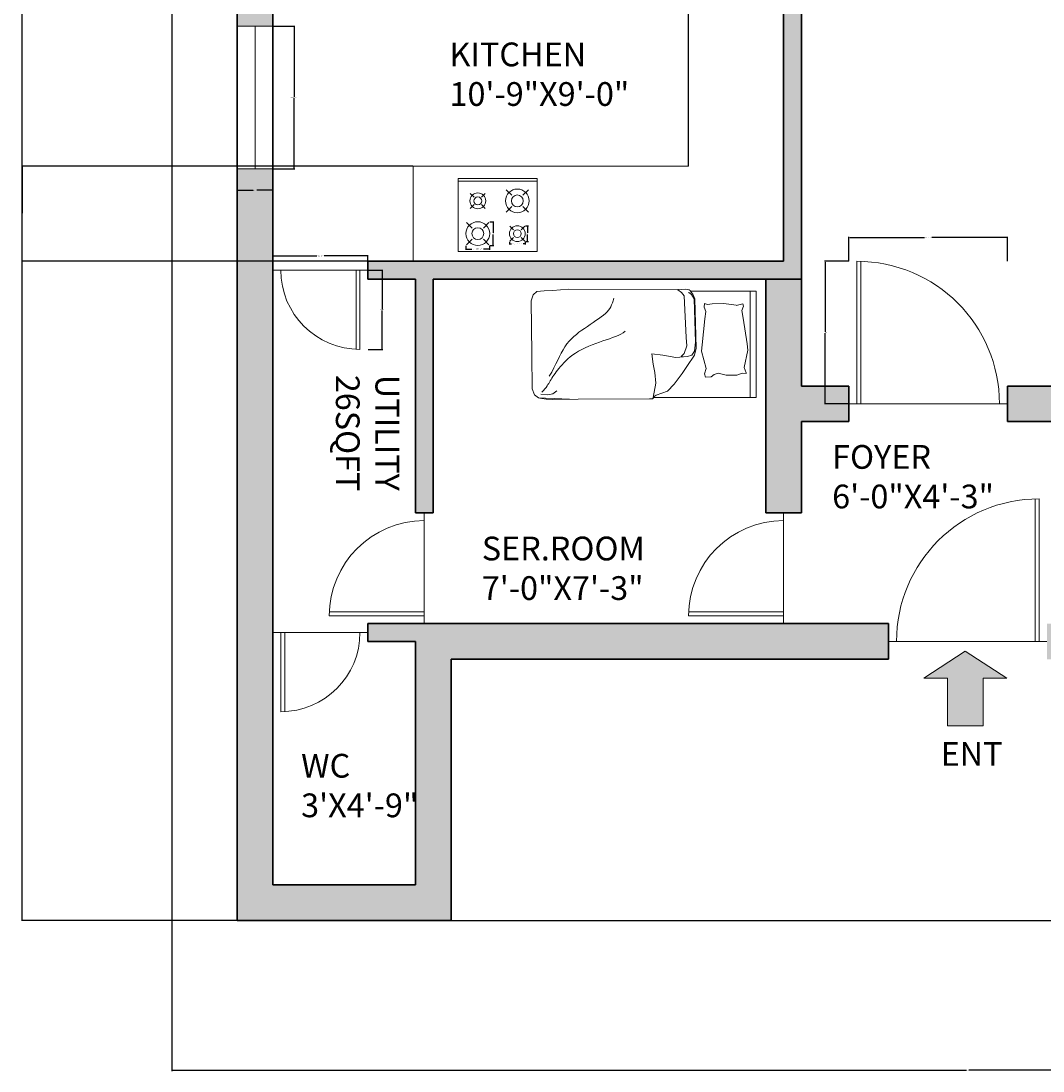
# Model space of a CAD drawing. Units: inches. Extents: x -36 to 442, y -676 to 151.
# Tile 1 of 8: x -36 to 222, y -676 to -411. Entities that reach past the tile are written whole.
import ezdxf

# ---------------------------------------------------------------- set-up
doc = ezdxf.new("R2010")
doc.units = ezdxf.units.IN
doc.header["$MEASUREMENT"] = 0
for name, color, linetype, lineweight in [('A-ANNO-DIMS', 2, 'Continuous', 18), ('A-ANNO-SYMB', 7, 'Continuous', 18), ('A-ANNO-TEXT', 7, 'Continuous', 18), ('A-AREA-IDEN', 7, 'Continuous', 18), ('A-DOOR', 4, 'Continuous', 18), ('A-EQPM', 8, 'Continuous', 18), ('A-FLOR-CASE', 32, 'Continuous', 18), ('A-FURN', 9, 'Continuous', 13), ('A-GLAZ', 4, 'Continuous', 13), ('A-WALL', 7, 'Continuous', 35), ('A-WALL-PATT', 8, 'Continuous', 13)]:
    doc.layers.add(name, color=color, linetype=linetype, lineweight=lineweight)
doc.styles.get("Standard").update_dxf_attribs({"font": 'arial.ttf'})
doc.dimstyles.get("Standard").update_dxf_attribs({"dimtxt": 0.18, "dimasz": 0.18, "dimexe": 0.18, "dimexo": 0.0625, "dimgap": 0.09, "dimtad": 0, "dimtih": 1, "dimtoh": 1, "dimdec": 0, "dimzin": 0, "dimdsep": 46, "dimlunit": 3, "dimtxsty": 'Standard', "dimcen": 0.09, "dimadec": 0, "dimazin": 0, "dimtfac": 1, "dimtdec": 0, "dimtofl": 0, "dimtmove": 0, "dimatfit": 3, "dimfxl": 1, "dimtolj": 1, "dimtzin": 0, "dimarcsym": 0})

# ---------------------------------------------------------------- blocks, each defined once
blk = doc.blocks.new('DOOR-SWING-24IN')
for p, q in [((24, 26), (24, 28)), ((24, 26), (24, 2)), ((24, 3), (0, 3)), ((24, 2), (0, 2)), ((24, 0), (24, 2))]:
    blk.add_line(p, q)
blk.add_arc((24, 2), 24, 90, 180)
blk = doc.blocks.new('DOOR-SWING-36IN')
for p, q in [((2, 0), (2, 36)), ((3, 0), (3, 36)), ((0, 0), (2, 0)), ((2, 0), (3, 0)), ((3, 0), (38, 0)), ((38, 0), (40, 0))]:
    blk.add_line(p, q)
blk.add_arc((2, 0), 36, 0, 90)
blk = doc.blocks.new('DOOR-SWING-20IN')
for p, q in [((0, 20), (2, 20)), ((2, 20), (2, 0)), ((2, 20), (22, 20)), ((3, 20), (3, 0)), ((24, 20), (22, 20))]:
    blk.add_line(p, q)
blk.add_arc((2, 20), 20, 270, 0)
blk = doc.blocks.new('GLAZING-UNIT-36IN')
for p, q in [((0, 36), (0, 0)), ((4.5, 36), (4.5, 0)), ((9, 0), (9, 36))]:
    blk.add_line(p, q)
blk = doc.blocks.new('COOKTOP-BURNER-LARGE')
for p, q in [((1.58, 4.41), (0.17, 5.82)), ((4.41, 4.41), (5.82, 5.82)), ((1.58, 1.58), (0.17, 0.17)), ((4.41, 1.58), (5.82, 0.17))]:
    blk.add_line(p, q)
blk.add_circle((3, 3), 3)
for start, end in [(0, 180), (180, 0)]:
    blk.add_arc((3, 3), 1.5, start, end)
blk = doc.blocks.new('COOKTOP-BURNER-SMALL')
for p, q in [((1.06, 2.94), (0.11, 3.88)), ((2.94, 2.94), (3.88, 3.88)), ((1.06, 1.06), (0.11, 0.11)), ((2.94, 1.06), (3.88, 0.11))]:
    blk.add_line(p, q)
blk.add_circle((2, 2), 2)
for start, end in [(0, 180), (180, 0)]:
    blk.add_arc((2, 2), 0.999, start, end)
blk = doc.blocks.new('*D19')
at = {"layer": 'A-ANNO-DIMS', "color": 0, "lineweight": -2, "transparency": 16777216}
for p, q in [((173.24, -471.43), (173.24, -465.32)), ((173.42, -465.5), (192.3, -465.5)), ((213.06, -465.5), (194.17, -465.5)), ((213.24, -471.43), (213.24, -465.32))]:
    blk.add_line(p, q, dxfattribs=at)
at = {"layer": 'A-ANNO-DIMS', "color": 0, "transparency": 16777216}
for points in [[(173.42, -465.47), (173.42, -465.53), (173.24, -465.5)], [(213.06, -465.47), (213.06, -465.53), (213.24, -465.5)]]:
    blk.add_solid(points, dxfattribs=at)
at = {"layer": 'Defpoints', "color": 0, "transparency": 16777216}
for p in [(213.24, -465.5), (173.24, -471.5), (213.24, -471.5)]:
    blk.add_point(p, dxfattribs=at)
at = {"layer": 'A-ANNO-DIMS', "color": 0, "transparency": 16777216, "insert": (193.24, -465.5), "char_height": 0.18, "attachment_point": 5}
blk.add_mtext('\\A1;DOOR 40 TYP.', dxfattribs=at)
blk = doc.blocks.new('*D20')
at = {"layer": 'A-ANNO-DIMS', "color": 0, "lineweight": -2, "transparency": 16777216}
for p, q in [((173.17, -471.5), (167.06, -471.5)), ((167.24, -471.68), (167.24, -489.32)), ((167.24, -507.32), (167.24, -489.68)), ((173.17, -507.5), (167.06, -507.5))]:
    blk.add_line(p, q, dxfattribs=at)
at = {"layer": 'A-ANNO-DIMS', "color": 0, "transparency": 16777216}
for points in [[(167.21, -471.68), (167.27, -471.68), (167.24, -471.5)], [(167.21, -507.32), (167.27, -507.32), (167.24, -507.5)]]:
    blk.add_solid(points, dxfattribs=at)
at = {"layer": 'Defpoints', "color": 0, "transparency": 16777216}
for p in [(167.24, -471.5), (173.24, -471.5), (173.24, -507.5)]:
    blk.add_point(p, dxfattribs=at)
at = {"layer": 'A-ANNO-DIMS', "color": 0, "transparency": 16777216, "insert": (167.24, -489.5), "char_height": 0.18, "attachment_point": 5}
blk.add_mtext('\\A1;36 TYP.', dxfattribs=at)
blk = doc.blocks.new('*D21')
at = {"layer": 'A-ANNO-DIMS', "color": 0, "lineweight": -2, "transparency": 16777216}
for p, q in [((27.74, -473.68), (27.74, -469.97)), ((27.92, -470.15), (38.8, -470.15)), ((51.56, -470.15), (40.67, -470.15)), ((51.74, -473.68), (51.74, -469.97))]:
    blk.add_line(p, q, dxfattribs=at)
at = {"layer": 'A-ANNO-DIMS', "color": 0, "transparency": 16777216}
for points in [[(27.92, -470.12), (27.92, -470.18), (27.74, -470.15)], [(51.56, -470.12), (51.56, -470.18), (51.74, -470.15)]]:
    blk.add_solid(points, dxfattribs=at)
at = {"layer": 'Defpoints', "color": 0, "transparency": 16777216}
for p in [(27.74, -470.15), (27.74, -473.75), (51.74, -473.75)]:
    blk.add_point(p, dxfattribs=at)
at = {"layer": 'A-ANNO-DIMS', "color": 0, "transparency": 16777216, "insert": (39.74, -470.15), "char_height": 0.18, "attachment_point": 5}
blk.add_mtext('\\A1;DOOR 24 TYP.', dxfattribs=at)
blk = doc.blocks.new('*D22')
at = {"layer": 'A-ANNO-DIMS', "color": 0, "lineweight": -2, "transparency": 16777216}
for p, q in [((51.8, -473.75), (55.52, -473.75)), ((55.34, -473.93), (55.34, -483.57)), ((55.34, -493.57), (55.34, -483.93)), ((51.8, -493.75), (55.52, -493.75))]:
    blk.add_line(p, q, dxfattribs=at)
at = {"layer": 'A-ANNO-DIMS', "color": 0, "transparency": 16777216}
for points in [[(55.31, -473.93), (55.37, -473.93), (55.34, -473.75)], [(55.31, -493.57), (55.37, -493.57), (55.34, -493.75)]]:
    blk.add_solid(points, dxfattribs=at)
at = {"layer": 'Defpoints', "color": 0, "transparency": 16777216}
for p in [(51.74, -473.75), (55.34, -473.75), (51.74, -493.75)]:
    blk.add_point(p, dxfattribs=at)
at = {"layer": 'A-ANNO-DIMS', "color": 0, "transparency": 16777216, "insert": (55.34, -483.75), "char_height": 0.18, "attachment_point": 5}
blk.add_mtext('\\A1;20 TYP.', dxfattribs=at)
blk = doc.blocks.new('*D23')
at = {"layer": 'A-ANNO-DIMS', "color": 0, "lineweight": -2, "transparency": 16777216}
for p, q in [((27.8, -412.15), (33.32, -412.15)), ((33.14, -412.33), (33.14, -429.97)), ((33.14, -447.97), (33.14, -430.33)), ((27.8, -448.15), (33.32, -448.15))]:
    blk.add_line(p, q, dxfattribs=at)
at = {"layer": 'A-ANNO-DIMS', "color": 0, "transparency": 16777216}
for points in [[(33.11, -412.33), (33.17, -412.33), (33.14, -412.15)], [(33.11, -447.97), (33.17, -447.97), (33.14, -448.15)]]:
    blk.add_solid(points, dxfattribs=at)
at = {"layer": 'Defpoints', "color": 0, "transparency": 16777216}
for p in [(27.74, -412.15), (33.14, -412.15), (27.74, -448.15)]:
    blk.add_point(p, dxfattribs=at)
at = {"layer": 'A-ANNO-DIMS', "color": 0, "transparency": 16777216, "insert": (33.14, -430.15), "char_height": 0.18, "attachment_point": 5}
blk.add_mtext('\\A1;WINDOW 36 TYP.', dxfattribs=at)
blk = doc.blocks.new('*D24')
at = {"layer": 'A-ANNO-DIMS', "color": 0, "lineweight": -2, "transparency": 16777216}
for p, q in [((18.74, -448.21), (18.74, -453.73)), ((27.74, -448.21), (27.74, -453.73)), ((18.92, -453.55), (22.78, -453.55)), ((27.56, -453.55), (23.69, -453.55))]:
    blk.add_line(p, q, dxfattribs=at)
at = {"layer": 'A-ANNO-DIMS', "color": 0, "transparency": 16777216}
for points in [[(18.92, -453.52), (18.92, -453.58), (18.74, -453.55)], [(27.56, -453.52), (27.56, -453.58), (27.74, -453.55)]]:
    blk.add_solid(points, dxfattribs=at)
at = {"layer": 'Defpoints', "color": 0, "transparency": 16777216}
for p in [(18.74, -448.15), (27.74, -448.15), (27.74, -453.55)]:
    blk.add_point(p, dxfattribs=at)
at = {"layer": 'A-ANNO-DIMS', "color": 0, "transparency": 16777216, "insert": (23.24, -453.55), "char_height": 0.18, "attachment_point": 5}
blk.add_mtext('\\A1;9 TYP.', dxfattribs=at)
blk = doc.blocks.new('*D33')
at = {"layer": 'A-ANNO-DIMS', "color": 0, "lineweight": -2, "transparency": 16777216}
for p, q in [((76.5, -467.57), (76.5, -468.59)), ((76.68, -468.41), (78.01, -468.41)), ((82.31, -468.41), (80.97, -468.41)), ((82.49, -467.57), (82.49, -468.59))]:
    blk.add_line(p, q, dxfattribs=at)
at = {"layer": 'A-ANNO-DIMS', "color": 0, "transparency": 16777216}
for points in [[(76.68, -468.38), (76.68, -468.44), (76.5, -468.41)], [(82.31, -468.38), (82.31, -468.44), (82.49, -468.41)]]:
    blk.add_solid(points, dxfattribs=at)
at = {"layer": 'Defpoints', "color": 0, "transparency": 16777216}
for p in [(76.5, -467.51), (82.49, -467.51), (82.49, -468.41)]:
    blk.add_point(p, dxfattribs=at)
at = {"layer": 'A-ANNO-DIMS', "color": 0, "transparency": 16777216, "insert": (79.49, -468.41), "char_height": 0.18, "attachment_point": 5}
blk.add_mtext('\\A1;LARGE BURNER 6 TYP.', dxfattribs=at)
blk = doc.blocks.new('*D34')
at = {"layer": 'A-ANNO-DIMS', "color": 0, "lineweight": -2, "transparency": 16777216}
for p, q in [((82.55, -461.52), (83.57, -461.52)), ((83.39, -461.7), (83.39, -464.33)), ((83.39, -467.33), (83.39, -464.7)), ((82.55, -467.51), (83.57, -467.51))]:
    blk.add_line(p, q, dxfattribs=at)
at = {"layer": 'A-ANNO-DIMS', "color": 0, "transparency": 16777216}
for points in [[(83.36, -461.7), (83.42, -461.7), (83.39, -461.52)], [(83.36, -467.33), (83.42, -467.33), (83.39, -467.51)]]:
    blk.add_solid(points, dxfattribs=at)
at = {"layer": 'Defpoints', "color": 0, "transparency": 16777216}
for p in [(82.49, -461.52), (83.39, -461.52), (82.49, -467.51)]:
    blk.add_point(p, dxfattribs=at)
at = {"layer": 'A-ANNO-DIMS', "color": 0, "transparency": 16777216, "insert": (83.39, -464.52), "char_height": 0.18, "attachment_point": 5}
blk.add_mtext('\\A1;6 TYP.', dxfattribs=at)
blk = doc.blocks.new('*D35')
at = {"layer": 'A-ANNO-DIMS', "color": 0, "lineweight": -2, "transparency": 16777216}
for p, q in [((87.48, -466.58), (87.48, -467.29)), ((91.48, -466.58), (91.48, -467.29)), ((87.66, -467.11), (88.01, -467.11)), ((91.3, -467.11), (90.95, -467.11))]:
    blk.add_line(p, q, dxfattribs=at)
at = {"layer": 'A-ANNO-DIMS', "color": 0, "transparency": 16777216}
for points in [[(87.66, -467.08), (87.66, -467.14), (87.48, -467.11)], [(91.3, -467.08), (91.3, -467.14), (91.48, -467.11)]]:
    blk.add_solid(points, dxfattribs=at)
at = {"layer": 'Defpoints', "color": 0, "transparency": 16777216}
for p in [(87.48, -466.51), (91.48, -466.51), (87.48, -467.11)]:
    blk.add_point(p, dxfattribs=at)
at = {"layer": 'A-ANNO-DIMS', "color": 0, "transparency": 16777216, "insert": (89.48, -467.11), "char_height": 0.18, "attachment_point": 5}
blk.add_mtext('\\A1;SMALL BURNER 4 TYP.', dxfattribs=at)
blk = doc.blocks.new('*D36')
at = {"layer": 'A-ANNO-DIMS', "color": 0, "lineweight": -2, "transparency": 16777216}
for p, q in [((91.54, -462.52), (92.26, -462.52)), ((92.08, -462.7), (92.08, -464.34)), ((91.54, -466.51), (92.26, -466.51)), ((92.08, -466.33), (92.08, -464.7))]:
    blk.add_line(p, q, dxfattribs=at)
at = {"layer": 'A-ANNO-DIMS', "color": 0, "transparency": 16777216}
for points in [[(92.05, -462.7), (92.11, -462.7), (92.08, -462.52)], [(92.05, -466.33), (92.11, -466.33), (92.08, -466.51)]]:
    blk.add_solid(points, dxfattribs=at)
at = {"layer": 'Defpoints', "color": 0, "transparency": 16777216}
for p in [(91.48, -462.52), (91.48, -466.51), (92.08, -466.51)]:
    blk.add_point(p, dxfattribs=at)
at = {"layer": 'A-ANNO-DIMS', "color": 0, "transparency": 16777216, "insert": (92.08, -464.52), "char_height": 0.18, "attachment_point": 5}
blk.add_mtext('\\A1;4 TYP.', dxfattribs=at)
blk = doc.blocks.new('*D49')
at = {"layer": 'A-ANNO-DIMS', "color": 0, "lineweight": -2, "transparency": 16777216}
for p, q in [((2.24, -363.56), (2.24, -675.98)), ((404.24, -512.06), (404.24, -675.98)), ((2.42, -675.8), (202.94, -675.8)), ((404.06, -675.8), (203.53, -675.8))]:
    blk.add_line(p, q, dxfattribs=at)
at = {"layer": 'A-ANNO-DIMS', "color": 0, "transparency": 16777216}
for points in [[(2.42, -675.77), (2.42, -675.83), (2.24, -675.8)], [(404.06, -675.77), (404.06, -675.83), (404.24, -675.8)]]:
    blk.add_solid(points, dxfattribs=at)
at = {"layer": 'Defpoints', "color": 0, "transparency": 16777216}
for p in [(2.24, -363.5), (404.24, -512), (404.24, -675.8)]:
    blk.add_point(p, dxfattribs=at)
at = {"layer": 'A-ANNO-DIMS', "color": 0, "transparency": 16777216, "insert": (203.24, -675.8), "char_height": 0.18, "attachment_point": 5}
blk.add_mtext('\\A1;402', dxfattribs=at)
blk = doc.blocks.new('*D50')
at = {"layer": 'A-ANNO-DIMS', "color": 0, "lineweight": -2, "transparency": 16777216}
for p, q in [((97.44, 113.5), (-35.74, 113.5)), ((-35.56, 113.32), (-35.56, -262.07)), ((-35.56, -637.82), (-35.56, -262.43)), ((18.67, -638), (-35.74, -638))]:
    blk.add_line(p, q, dxfattribs=at)
at = {"layer": 'A-ANNO-DIMS', "color": 0, "transparency": 16777216}
for points in [[(-35.59, 113.32), (-35.53, 113.32), (-35.56, 113.5)], [(-35.59, -637.82), (-35.53, -637.82), (-35.56, -638)]]:
    blk.add_solid(points, dxfattribs=at)
at = {"layer": 'Defpoints', "color": 0, "transparency": 16777216}
for p in [(-35.56, 113.5), (97.5, 113.5), (18.74, -638)]:
    blk.add_point(p, dxfattribs=at)
at = {"layer": 'A-ANNO-DIMS', "color": 0, "transparency": 16777216, "insert": (-35.56, -262.25), "char_height": 0.18, "attachment_point": 5}
blk.add_mtext('\\A1;751.5', dxfattribs=at)
blk = doc.blocks.new('*D61')
at = {"layer": 'A-ANNO-DIMS', "color": 0, "lineweight": -2, "transparency": 16777216}
for p, q in [((242.3, -572), (442.22, -572)), ((442.04, -572.18), (442.04, -604.82)), ((442.04, -637.82), (442.04, -605.18)), ((72.8, -638), (442.22, -638))]:
    blk.add_line(p, q, dxfattribs=at)
at = {"layer": 'A-ANNO-DIMS', "color": 0, "transparency": 16777216}
for points in [[(442.01, -572.18), (442.07, -572.18), (442.04, -572)], [(442.01, -637.82), (442.07, -637.82), (442.04, -638)]]:
    blk.add_solid(points, dxfattribs=at)
at = {"layer": 'Defpoints', "color": 0, "transparency": 16777216}
for p in [(242.24, -572), (442.04, -572), (72.74, -638)]:
    blk.add_point(p, dxfattribs=at)
at = {"layer": 'A-ANNO-DIMS', "color": 0, "transparency": 16777216, "insert": (442.04, -605), "char_height": 0.18, "attachment_point": 5}
blk.add_mtext('\\A1;66', dxfattribs=at)
blk = doc.blocks.new('*D62')
at = {"layer": 'A-ANNO-DIMS', "color": 0, "lineweight": -2, "transparency": 16777216}
for p, q in [((63.1, -447.5), (-35.74, -447.5)), ((-35.56, -447.68), (-35.56, -459.32)), ((-35.56, -471.32), (-35.56, -459.68)), ((63.1, -471.5), (-35.74, -471.5))]:
    blk.add_line(p, q, dxfattribs=at)
at = {"layer": 'A-ANNO-DIMS', "color": 0, "transparency": 16777216}
for points in [[(-35.59, -447.68), (-35.53, -447.68), (-35.56, -447.5)], [(-35.59, -471.32), (-35.53, -471.32), (-35.56, -471.5)]]:
    blk.add_solid(points, dxfattribs=at)
at = {"layer": 'Defpoints', "color": 0, "transparency": 16777216}
for p in [(63.16, -447.5), (-35.56, -471.5), (63.16, -471.5)]:
    blk.add_point(p, dxfattribs=at)
at = {"layer": 'A-ANNO-DIMS', "color": 0, "transparency": 16777216, "insert": (-35.56, -459.5), "char_height": 0.18, "attachment_point": 5}
blk.add_mtext('\\A1;24', dxfattribs=at)
blk = doc.blocks.new('*D63')
at = {"layer": 'A-ANNO-DIMS', "color": 0, "lineweight": -2, "transparency": 16777216}
for p, q in [((132.74, -447.43), (132.74, 151.48)), ((132.92, 151.3), (144.51, 151.3)), ((156.56, 151.3), (144.96, 151.3)), ((156.74, -471.43), (156.74, 151.48))]:
    blk.add_line(p, q, dxfattribs=at)
at = {"layer": 'A-ANNO-DIMS', "color": 0, "transparency": 16777216}
for points in [[(132.92, 151.33), (132.92, 151.27), (132.74, 151.3)], [(156.56, 151.33), (156.56, 151.27), (156.74, 151.3)]]:
    blk.add_solid(points, dxfattribs=at)
at = {"layer": 'Defpoints', "color": 0, "transparency": 16777216}
for p in [(156.74, 151.3), (132.74, -447.5), (156.74, -471.5)]:
    blk.add_point(p, dxfattribs=at)
at = {"layer": 'A-ANNO-DIMS', "color": 0, "transparency": 16777216, "insert": (144.74, 151.3), "char_height": 0.18, "attachment_point": 5}
blk.add_mtext('\\A1;24', dxfattribs=at)

msp = doc.modelspace()

# ---------------------------------------------------------------- hatches: boundary and pattern name
at = {"layer": 'A-ANNO-SYMB'}
h = msp.add_hatch(color=256, dxfattribs=at)
h.dxf.hatch_style = 1
h.paths.add_polyline_path([(207.111, -576.798), (213.111, -576.798), (202.611, -569.981), (192.111, -576.798), (198.111, -576.798), (198.111, -588.798), (207.111, -588.798)])
at = {"layer": 'A-WALL-PATT'}
h = msp.add_hatch(color=256, dxfattribs=at)
h.dxf.hatch_style = 1
h.paths.add_polyline_path([(288, 113.503), (193.5, 113.503), (97.5, 113.503), (97.5, 104.864), (106.5, 104.864), (106.5, 104.503), (193.5, 104.503), (193.5, 5.503), (193.5, 1.003), (213.735, 1.003), (213.735, -135.497), (218.235, -135.497), (218.235, 1.003), (251, 1.003), (251, 3.253), (251, 5.503), (198, 5.503), (198, 104.503), (279, 104.503), (279, 104.209), (288, 104.209)])
h.paths.add_polyline_path([(378.735, 81.646), (362.235, 81.646), (288, 81.646), (288, 80.209), (279, 80.209), (279, 5.503), (279, 1.003), (353.235, 1.003), (353.235, 0.242), (362.235, 0.242), (362.235, 5.503), (288, 5.503), (288, 77.146), (362.235, 77.146), (374.235, 77.146), (374.235, 5.503), (362.235, 5.503), (362.235, 1.003), (374.235, 1.003), (378.735, 1.003), (378.735, 5.503), (378.735, 77.146)])
h.paths.add_polyline_path([(362.235, -35.758), (353.235, -35.758), (353.235, -196.997), (218.235, -196.997), (213.735, -196.997), (213.735, -205.997), (218.235, -205.997), (378.735, -205.997), (378.735, -205.779), (387.735, -205.779), (387.735, -202.472), (387.735, -196.997), (378.735, -196.997), (362.235, -196.997)])
h.paths.add_polyline_path([(218.235, -175.497), (215.985, -175.497), (213.735, -175.497), (213.735, -196.997), (218.235, -196.997)], flags=17)
h.paths.add_polyline_path([(158.235, -201.497), (98.235, -201.497), (98.235, -205.997), (158.235, -205.997)])
h.paths.add_polyline_path([(173.735, -130.997), (27.735, -130.997), (27.735, -35.267), (18.735, -35.267), (18.735, -138.68), (27.735, -138.68), (27.735, -135.497), (93.735, -135.497), (93.735, -201.497), (98.235, -201.497), (98.235, -135.497), (158.235, -135.497), (158.235, -173.497), (160.739, -173.497), (162.735, -173.497), (162.735, -135.497), (173.735, -135.497), (173.735, -133.017)])
h.paths.add_polyline_path([(98.235, -201.497), (93.735, -201.497), (93.735, -205.997), (98.235, -205.997)])
h.paths.add_polyline_path([(162.735, -201.497), (158.235, -201.497), (158.235, -205.997), (162.735, -205.997)])
h.paths.add_polyline_path([(63.735, -205.997), (63.735, -201.497), (27.735, -201.497), (27.735, -162.68), (18.735, -162.68), (18.735, -210.497), (63.735, -210.497)])
h.paths.add_polyline_path([(65.735, -203.604), (65.735, -201.497), (63.735, -201.497), (63.735, -205.997), (65.735, -205.997)])
h.paths.add_polyline_path([(165.5, 5.503), (106.5, 5.503), (106.5, 80.864), (97.5, 80.864), (97.5, 81.646), (6.735, 81.646), (2.235, 81.646), (2.235, 77.146), (2.235, 5.503), (2.235, 1.003), (6.735, 1.003), (18.735, 1.003), (18.735, 5.503), (6.735, 5.503), (6.735, 77.146), (97.5, 77.146), (97.5, 5.503), (18.735, 5.503), (18.735, 0.733), (27.735, 0.733), (27.735, 1.003), (165.5, 1.003), (165.5, 3.253)])
h.paths.add_polyline_path([(18.735, -201.497), (6.735, -201.497), (2.235, -201.497), (2.235, -210.497), (2.235, -354.497), (2.235, -363.497), (6.735, -363.497), (18.735, -363.497), (18.735, -358.997), (18.735, -354.497), (6.735, -354.497), (6.735, -210.497), (18.735, -210.497)])
h.paths.add_polyline_path([(63.735, -210.497), (54.735, -210.497), (54.735, -240.747), (63.735, -240.747)])
h.paths.add_polyline_path([(63.735, -336.747), (54.735, -336.747), (54.735, -354.497), (18.735, -354.497), (18.735, -358.997), (18.735, -363.497), (104.735, -363.497), (104.735, -361.247), (104.735, -358.997), (63.735, -358.997)])
h.paths.add_polyline_path([(27.735, -448.151), (18.735, -448.151), (18.735, -637.997), (72.735, -637.997), (72.735, -571.997), (183.235, -571.997), (183.235, -562.997), (57.197, -562.997), (51.735, -562.997), (51.735, -567.497), (57.197, -567.497), (63.735, -567.497), (63.735, -571.997), (63.735, -628.997), (27.735, -628.997), (27.735, -475.997), (27.735, -471.497)])
h.paths.add_polyline_path([(27.735, -363.497), (18.735, -363.497), (18.735, -412.151), (27.735, -412.151)])
h.paths.add_polyline_path([(161.235, -358.997), (132.735, -358.997), (132.735, -363.497), (156.735, -363.497), (156.735, -471.497), (51.735, -471.497), (51.735, -475.997), (63.735, -475.997), (63.735, -534.997), (65.985, -534.997), (68.235, -534.997), (68.235, -475.997), (161.235, -475.997)])
h.paths.add_polyline_path([(161.235, -511.997), (173.235, -511.997), (173.235, -502.997), (161.235, -502.997), (161.235, -475.997), (152.235, -475.997), (152.235, -534.997), (156.735, -534.997), (161.235, -534.997)], flags=17)
h.paths.add_polyline_path([(362.235, -502.997), (353.235, -502.997), (213.235, -502.997), (213.235, -507.497), (213.235, -511.997), (362.235, -511.997)])
h.paths.add_polyline_path([(242.235, -548.019), (233.235, -548.019), (233.235, -562.997), (223.235, -562.997), (223.235, -567.497), (223.235, -571.997), (242.235, -571.997)])
h.paths.add_polyline_path([(404.235, -502.997), (399.735, -502.997), (362.235, -502.997), (362.235, -511.997), (399.735, -511.997), (404.235, -511.997)])
h.paths.add_polyline_path([(362.235, -482.123), (353.235, -482.123), (353.235, -502.997), (362.235, -502.997)])
h.paths.add_polyline_path([(404.235, -295.997), (404.235, -286.997), (387.735, -286.997), (387.735, -295.997), (399.735, -295.997), (399.735, -502.997), (404.235, -502.997)])
h.paths.add_polyline_path([(362.235, -355.863), (353.235, -355.863), (353.235, -386.123), (362.235, -386.123)])
h.paths.add_polyline_path([(387.735, -286.997), (378.735, -286.997), (213.735, -286.997), (213.735, -295.997), (353.235, -295.997), (353.235, -295.863), (362.235, -295.863), (362.235, -295.997), (378.735, -295.997), (387.735, -295.997)])
h.paths.add_polyline_path([(387.735, -241.779), (378.735, -241.779), (378.735, -286.997), (387.735, -286.997)])
h.paths.add_polyline_path([(387.735, -175.497), (362.235, -175.497), (362.235, -184.497), (387.735, -184.497)], flags=17)
h.paths.add_polyline_path([(387.735, -184.497), (383.235, -184.497), (383.235, -192.497), (378.735, -192.497), (366.735, -192.497), (366.735, -184.497), (362.235, -184.497), (362.235, -196.997), (378.735, -196.997), (387.735, -196.997)], flags=17)
h.paths.add_polyline_path([(240.604, 40.967), (282.575, 40.967), (282.575, 63.356), (240.604, 63.356)], flags=25)

# ---------------------------------------------------------------- linework, layer by layer
at = {"layer": 'A-ANNO-SYMB'}
for p, q in [((192.111, -576.798), (202.611, -569.981)), ((202.611, -569.981), (213.111, -576.798)), ((198.111, -576.798), (192.111, -576.798)), ((198.111, -576.798), (198.111, -588.798)), ((207.111, -588.798), (207.111, -576.798)), ((207.111, -576.798), (213.111, -576.798)), ((198.111, -588.798), (207.111, -588.798))]:
    msp.add_line(p, q, dxfattribs=at)
at = {"layer": 'A-DOOR'}
for p, q in [((220.235, -567.497), (220.235, -531.497)), ((221.235, -567.497), (221.235, -531.497)), ((65.985, -536.997), (65.985, -534.997)), ((65.985, -536.997), (65.985, -559.997)), ((65.985, -559.997), (41.985, -559.997)), ((65.985, -560.997), (41.985, -560.997)), ((65.985, -559.997), (65.985, -560.997)), ((65.985, -562.997), (65.985, -560.997)), ((183.235, -567.497), (185.235, -567.497)), ((185.235, -567.497), (220.235, -567.497)), ((220.235, -567.497), (223.235, -567.497))]:
    msp.add_line(p, q, dxfattribs=at)
for centre, radius in [((221.235, -567.497), 36), ((65.985, -560.997), 24)]:
    msp.add_arc(centre, radius, 90, 180, dxfattribs=at)
at = {"layer": 'A-EQPM'}
for p, q in [((74.499, -450.591), (94.473, -450.591)), ((74.499, -450.591), (74.499, -469.033)), ((94.473, -450.591), (94.473, -469.033)), ((74.499, -451.256), (94.473, -451.256)), ((74.499, -469.033), (94.473, -469.033))]:
    msp.add_line(p, q, dxfattribs=at)
at = {"layer": 'A-FLOR-CASE'}
for p, q in [((132.735, -363.497), (132.735, -446.014)), ((63.159, -471.497), (63.159, -447.497)), ((63.159, -447.497), (132.735, -447.497)), ((132.735, -447.497), (132.735, -446.014))]:
    msp.add_line(p, q, dxfattribs=at)
at = {"layer": 'A-FURN'}
for p, q in [((94.423, -479.163), (93.469, -479.95)), ((96.224, -478.964), (94.423, -479.163)), ((98.411, -478.85), (96.224, -478.964)), ((102.296, -478.514), (98.411, -478.85)), ((130.844, -478.58), (102.296, -478.514)), ((132.011, -478.562), (130.844, -478.58)), ((132.51, -478.609), (132.011, -478.562)), ((133.22, -479.062), (149.808, -479.062)), ((93.469, -479.95), (92.955, -481.476)), ((93.159, -494.899), (92.955, -481.476)), ((144.733, -482.667), (146.466, -482.206)), ((136.031, -494.211), (136.137, -492.579)), ((147.686, -493.951), (147.507, -492.325)), ((93.159, -494.899), (93.159, -498.737)), ((131.109, -495.655), (131.109, -495.295)), ((137.141, -498.564), (136.031, -494.211)), ((146.771, -498.349), (147.686, -493.951)), ((147.268, -499.704), (146.771, -498.349)), ((93.159, -498.737), (93.259, -500.096)), ((93.259, -500.096), (93.26, -503.679)), ((136.705, -499.94), (137.141, -498.564)), ((136.979, -500.783), (136.705, -499.94)), ((138.414, -500.697), (136.979, -500.783)), ((139.188, -500.098), (138.414, -500.697)), ((140.162, -499.757), (139.188, -500.098)), ((142.193, -500.248), (140.162, -499.757)), ((144.935, -500.272), (142.193, -500.248)), ((146.232, -499.73), (144.935, -500.272)), ((147.233, -499.832), (146.232, -499.73)), ((147.233, -499.832), (146.232, -499.73)), ((147.233, -499.832), (147.268, -499.704)), ((93.819, -505.189), (93.26, -503.679)), ((94.797, -505.947), (93.819, -505.189)), ((96.603, -506.091), (94.797, -505.947)), ((95.126, -506.039), (96.721, -506.341)), ((95.384, -505.082), (97.154, -505.208)), ((98.792, -506.139), (96.603, -506.091)), ((96.721, -506.341), (98.257, -506.433)), ((97.154, -505.208), (98.418, -504.955)), ((98.257, -506.433), (104.856, -506.319)), ((98.418, -504.955), (99.43, -504.197)), ((102.686, -506.357), (98.792, -506.139)), ((104.856, -506.319), (122.876, -506.268)), ((123.816, -505.841), (123.845, -505.906)), ((123.873, -505.895), (149.808, -505.895))]:
    msp.add_line(p, q, dxfattribs=at)
for points in [[(123.799, -505.896), (124.432, -502.288), (124.23, -499.624), (123.792, -497.448), (123.43, -494.868), (126.247, -495.216), (129.524, -495.795), (132.418, -495.54), (133.588, -495.163), (134.259, -494.219), (134.467, -491.953), (134.139, -480.983), (133.475, -479.862), (132.821, -479.387), (132.759, -479.327)], [(133.411, -479.334), (133.797, -479.776), (134.301, -480.981), (134.651, -493.405), (134.193, -495.19), (132.295, -498.047), (131.109, -499.843), (129.127, -502.54), (127.374, -504.263), (124.558, -505.276), (123.82, -505.775)], [(130.819, -495.579), (131.642, -494.772), (132.259, -492.875), (132.134, -490.758), (131.606, -480.246), (130.94, -479.359), (130.044, -478.691)], [(132.541, -478.625), (132.876, -478.729), (133.134, -478.881), (133.22, -479.062), (133.405, -479.272), (133.416, -479.303)], [(148.317, -505.895), (148.317, -479.062)], [(149.808, -479.062), (149.808, -505.895)], [(97.533, -500.534), (98.158, -499.46), (98.715, -498.419), (99.22, -497.415), (99.688, -496.451), (100.134, -495.531), (100.573, -494.659), (101.022, -493.838), (101.495, -493.071), (102.004, -492.361), (102.55, -491.702), (103.13, -491.087), (103.742, -490.509), (104.382, -489.961), (105.048, -489.437), (105.737, -488.928), (106.447, -488.429), (107.173, -487.933), (107.904, -487.441), (108.629, -486.954), (109.334, -486.475), (110.007, -486.005), (110.637, -485.547), (111.21, -485.101), (111.715, -484.671), (112.143, -484.255), (112.501, -483.844), (112.801, -483.427), (113.056, -482.991), (113.275, -482.525), (113.472, -482.017), (113.658, -481.455), (113.843, -480.829)], [(136.137, -492.579), (136.821, -486.048), (137.053, -484.153), (136.645, -483.051), (136.762, -482.136), (137.483, -482.386), (138.721, -482.236), (141.593, -482.193), (144.732, -482.602)], [(147.507, -492.325), (146.532, -485.831), (146.215, -483.948), (146.574, -482.829), (146.466, -482.206)], [(95.637, -504.576), (96.071, -504.125), (96.435, -503.714), (96.74, -503.335), (96.998, -502.982), (97.222, -502.646), (97.423, -502.32), (97.614, -501.998), (97.807, -501.671), (98.012, -501.333), (98.232, -500.983), (98.47, -500.619), (98.726, -500.239), (99.004, -499.845), (99.304, -499.433), (99.628, -499.003), (99.978, -498.555), (100.356, -498.088), (100.766, -497.606), (101.214, -497.114), (101.703, -496.616), (102.239, -496.117), (102.825, -495.621), (103.468, -495.134), (104.171, -494.66), (104.936, -494.204), (105.755, -493.766), (106.614, -493.347), (107.502, -492.95), (108.406, -492.574), (109.314, -492.221), (110.214, -491.892), (111.093, -491.587), (111.942, -491.306), (112.755, -491.04), (113.531, -490.778), (114.266, -490.51), (114.958, -490.226), (115.605, -489.914), (116.203, -489.564), (116.751, -489.166)], [(122.924, -506.267), (123.619, -506.217), (123.828, -506.013), (123.873, -505.895)]]:
    msp.add_lwpolyline(points, dxfattribs=at)
at = {"layer": 'A-GLAZ'}
for p, q in [((27.735, -412.151), (18.735, -412.151)), ((18.735, -448.151), (27.735, -448.151))]:
    msp.add_line(p, q, dxfattribs=at)
at = {"layer": 'A-WALL'}
for p, q in [((18.735, -358.997), (18.735, -637.997)), ((161.235, -358.997), (161.235, -502.997)), ((27.735, -363.497), (27.735, -471.497)), ((156.735, -363.497), (156.735, -471.497)), ((27.735, -471.497), (27.735, -475.997)), ((51.735, -471.497), (156.735, -471.497)), ((51.735, -475.997), (51.735, -471.497)), ((27.735, -475.997), (27.735, -628.997)), ((51.735, -475.997), (63.735, -475.997)), ((63.735, -475.997), (63.735, -534.997)), ((68.235, -475.997), (68.235, -534.997)), ((68.235, -475.997), (161.235, -475.997)), ((152.235, -475.997), (152.235, -534.997)), ((161.235, -502.997), (173.235, -502.997)), ((173.235, -502.997), (173.235, -511.997)), ((213.235, -507.497), (213.235, -502.997)), ((213.235, -502.997), (353.235, -502.997)), ((213.235, -507.497), (213.235, -511.997)), ((161.235, -511.997), (173.235, -511.997)), ((161.235, -511.997), (161.235, -534.997)), ((213.235, -511.997), (362.235, -511.997)), ((65.985, -534.997), (63.735, -534.997)), ((65.985, -534.997), (68.235, -534.997)), ((156.735, -534.997), (152.235, -534.997)), ((156.735, -534.997), (161.235, -534.997)), ((51.735, -567.497), (51.735, -562.997)), ((51.735, -562.997), (57.197, -562.997)), ((57.197, -562.997), (183.235, -562.997)), ((152.235, -562.997), (161.235, -562.997)), ((183.235, -562.997), (183.235, -571.997)), ((51.735, -567.497), (57.197, -567.497)), ((57.197, -567.497), (63.735, -567.497)), ((63.735, -567.497), (63.735, -571.997)), ((63.735, -571.997), (63.735, -628.997)), ((72.735, -571.997), (72.735, -637.997)), ((72.735, -571.997), (183.235, -571.997)), ((27.735, -628.997), (63.735, -628.997)), ((18.735, -637.997), (72.735, -637.997))]:
    msp.add_line(p, q, dxfattribs=at)

# ---------------------------------------------------------------- block references
at = {"layer": 'A-DOOR'}
for name, p in [('DOOR-SWING-36IN', (173.235, -507.497)), ('DOOR-SWING-24IN', (132.735, -562.997)), ('DOOR-SWING-20IN', (27.735, -585.247))]:
    msp.add_blockref(name, p, dxfattribs=at)
at = {"layer": 'A-DOOR', "extrusion": (0, 0, -1), "zscale": -1}
msp.add_blockref('DOOR-SWING-20IN', (-51.735, -493.747), dxfattribs=at)
at = {"layer": 'A-EQPM', "rotation": 180}
for name, p in [('COOKTOP-BURNER-LARGE', (92.476, -453.254)), ('COOKTOP-BURNER-SMALL', (91.477, -462.519))]:
    msp.add_blockref(name, p, dxfattribs=at)
at = {"layer": 'A-EQPM'}
for name, p in [('COOKTOP-BURNER-SMALL', (77.495, -458.247)), ('COOKTOP-BURNER-LARGE', (76.496, -467.512))]:
    msp.add_blockref(name, p, dxfattribs=at)
at = {"layer": 'A-GLAZ'}
msp.add_blockref('GLAZING-UNIT-36IN', (18.735, -448.151), dxfattribs=at)

# ---------------------------------------------------------------- texts
at = {"layer": 'A-ANNO-TEXT', "insert": (196.369, -592.904), "char_height": 6, "attachment_point": 1}
msp.add_mtext('ENT', dxfattribs=at)
at = {"layer": 'A-AREA-IDEN', "char_height": 6, "attachment_point": 1}
for s, insert in [('KITCHEN\\P10\'-9"X9\'-0"', (72.346, -416.255)), ('FOYER\\P6\'-0"X4\'-3"', (168.99, -517.898)), ('SER.ROOM\\P7\'-0"X7\'-3"', (80.51, -541.028)), ('WC\\P3\'X4\'-9"', (34.872, -595.889))]:
    msp.add_mtext(s, dxfattribs=dict(at, insert=insert))
at = {"layer": 'A-AREA-IDEN', "insert": (59.651, -500.164), "char_height": 6, "attachment_point": 1, "rotation": 270}
msp.add_mtext('UTILITY\\P26SQFT', dxfattribs=at)

# ---------------------------------------------------------------- dimensions: what is measured, and where the dimension line sits
at = {"layer": 'A-ANNO-DIMS'}
for base, p1, p2, picture, middle in [((156.735, 151.303), (132.735, -447.497), (156.735, -471.497), '*D63', (144.735, 151.303)), ((404.235, -675.797), (2.235, -363.497), (404.235, -511.997), '*D49', (203.235, -675.797))]:
    dim = msp.add_linear_dim(base=base, p1=p1, p2=p2, dimstyle='Standard', override={"dimdec": 0, "dimlfac": 1, "dimrnd": 0, "dimzin": 0, "dimdsep": 46, "dimlunit": 2}, dxfattribs=at)
    dim.commit()
    dim.dimension.update_dxf_attribs({"geometry": picture, "text_midpoint": middle})
for base, p1, p2, override, picture, middle in [((-35.565, 113.503), (18.735, -637.997), (97.5, 113.503), {"dimdec": 1, "dimlfac": 1, "dimrnd": 0, "dimzin": 0, "dimdsep": 46, "dimlunit": 2}, '*D50', (-35.565, -262.247)), ((-35.565, -471.497), (63.159, -447.497), (63.159, -471.497), {"dimdec": 0, "dimlfac": 1, "dimrnd": 0, "dimzin": 0, "dimdsep": 46, "dimlunit": 2}, '*D62', (-35.565, -459.497)), ((442.035, -571.997), (72.735, -637.997), (242.235, -571.997), {"dimdec": 0, "dimlfac": 1, "dimrnd": 0, "dimzin": 0, "dimdsep": 46, "dimlunit": 2}, '*D61', (442.035, -604.997))]:
    dim = msp.add_linear_dim(base=base, p1=p1, p2=p2, angle=90, dimstyle='Standard', override=override, dxfattribs=at)
    dim.commit()
    dim.dimension.update_dxf_attribs({"geometry": picture, "text_midpoint": middle})
for base, p1, p2, angle, text, picture, middle in [((33.135, -412.151), (27.735, -448.151), (27.735, -412.151), 90, 'WINDOW <> TYP.', '*D23', (33.135, -430.151)), ((83.387, -461.52), (82.488, -467.512), (82.488, -461.52), 90, '<> TYP.', '*D34', (83.387, -464.516)), ((92.076, -466.513), (91.477, -462.518), (91.477, -466.513), 270, '<> TYP.', '*D36', (92.076, -464.516)), ((87.482, -467.112), (91.477, -466.513), (87.482, -466.513), 180, 'SMALL BURNER <> TYP.', '*D35', (89.479, -467.112)), ((27.735, -470.147), (51.735, -473.747), (27.735, -473.747), 180, 'DOOR <> TYP.', '*D21', (39.735, -470.147)), ((167.235, -471.497), (173.235, -507.497), (173.235, -471.497), 90, '<> TYP.', '*D20', (167.235, -489.497)), ((55.335, -473.747), (51.735, -493.747), (51.735, -473.747), 90, '<> TYP.', '*D22', (55.335, -483.747))]:
    dim = msp.add_linear_dim(base=base, p1=p1, p2=p2, angle=angle, text=text, dimstyle='Standard', override={"dimdec": 0, "dimlfac": 1, "dimrnd": 0, "dimzin": 0, "dimdsep": 46, "dimlunit": 2}, dxfattribs=at)
    dim.commit()
    dim.dimension.update_dxf_attribs({"geometry": picture, "text_midpoint": middle})
for base, p1, p2, text, picture, middle in [((27.735, -453.551), (18.735, -448.151), (27.735, -448.151), '<> TYP.', '*D24', (23.235, -453.551)), ((213.235, -465.497), (173.235, -471.497), (213.235, -471.497), 'DOOR <> TYP.', '*D19', (193.235, -465.497)), ((82.488, -468.411), (76.496, -467.512), (82.488, -467.512), 'LARGE BURNER <> TYP.', '*D33', (79.492, -468.411))]:
    dim = msp.add_linear_dim(base=base, p1=p1, p2=p2, text=text, dimstyle='Standard', override={"dimdec": 0, "dimlfac": 1, "dimrnd": 0, "dimzin": 0, "dimdsep": 46, "dimlunit": 2}, dxfattribs=at)
    dim.commit()
    dim.dimension.update_dxf_attribs({"geometry": picture, "text_midpoint": middle})

doc.saveas('drawing.dxf')
